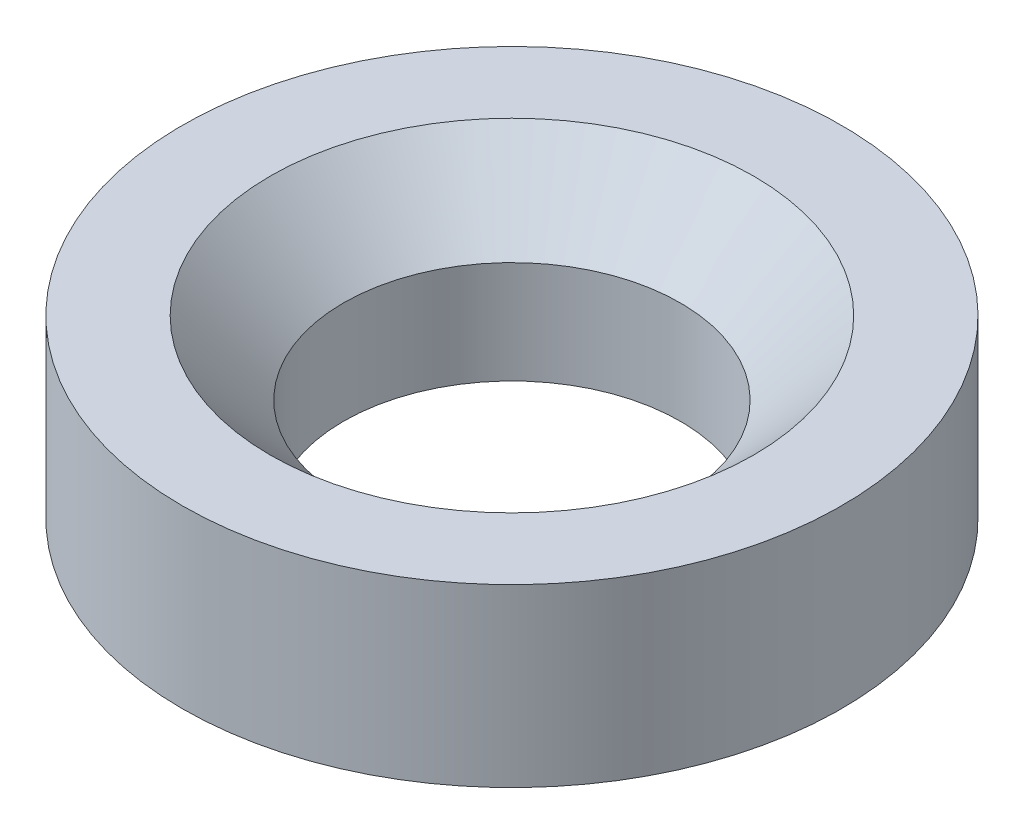
ISO-10303-21;
HEADER;
FILE_DESCRIPTION(('STEP AP214'),'2;1');
FILE_NAME('part.step','',(''),(''),'','','');
FILE_SCHEMA(('AUTOMOTIVE_DESIGN { 1 0 10303 214 1 1 1 1 }'));
ENDSEC;
DATA;
#1=APPLICATION_CONTEXT('core data for automotive mechanical design processes');
#2=APPLICATION_PROTOCOL_DEFINITION('international standard','automotive_design',2000,#1);
#3=PRODUCT_CONTEXT('',#1,'mechanical');
#4=PRODUCT('Part','Part','',(#3));
#5=PRODUCT_RELATED_PRODUCT_CATEGORY('part','',(#4));
#6=PRODUCT_DEFINITION_FORMATION('','',#4);
#7=PRODUCT_DEFINITION_CONTEXT('part definition',#1,'design');
#8=PRODUCT_DEFINITION('design','',#6,#7);
#9=PRODUCT_DEFINITION_SHAPE('','',#8);
#10=(LENGTH_UNIT() NAMED_UNIT(*) SI_UNIT(.MILLI.,.METRE.));
#11=(NAMED_UNIT(*) PLANE_ANGLE_UNIT() SI_UNIT($,.RADIAN.));
#12=(NAMED_UNIT(*) SI_UNIT($,.STERADIAN.) SOLID_ANGLE_UNIT());
#13=UNCERTAINTY_MEASURE_WITH_UNIT(LENGTH_MEASURE(1.E-05),#10,'distance_accuracy_value','');
#14=(GEOMETRIC_REPRESENTATION_CONTEXT(3) GLOBAL_UNCERTAINTY_ASSIGNED_CONTEXT((#13)) GLOBAL_UNIT_ASSIGNED_CONTEXT((#10,
#11,#12)) REPRESENTATION_CONTEXT('',''));
#15=CARTESIAN_POINT('',(0.,0.,0.));
#16=DIRECTION('',(0.,0.,1.));
#17=DIRECTION('',(1.,0.,0.));
#18=AXIS2_PLACEMENT_3D('',#15,#16,#17);
#19=CARTESIAN_POINT('',(0.,12.,0.));
#20=DIRECTION('',(0.,-1.,0.));
#21=DIRECTION('',(0.,0.,-1.));
#22=AXIS2_PLACEMENT_3D('',#19,#20,#21);
#23=CYLINDRICAL_SURFACE('',#22,22.5);
#24=CARTESIAN_POINT('',(0.,12.,0.));
#25=DIRECTION('',(0.,1.,0.));
#26=DIRECTION('',(0.,0.,1.));
#27=AXIS2_PLACEMENT_3D('',#24,#25,#26);
#28=CIRCLE('',#27,22.5);
#29=CARTESIAN_POINT('',(0.,12.,22.5));
#30=VERTEX_POINT('',#29);
#31=EDGE_CURVE('E10',#30,#30,#28,.T.);
#32=ORIENTED_EDGE('',*,*,#31,.F.);
#33=EDGE_LOOP('',(#32));
#34=FACE_BOUND('',#33,.T.);
#35=CARTESIAN_POINT('',(0.,0.,0.));
#36=DIRECTION('',(0.,1.,0.));
#37=DIRECTION('',(0.,0.,1.));
#38=AXIS2_PLACEMENT_3D('',#35,#36,#37);
#39=CIRCLE('',#38,22.5);
#40=CARTESIAN_POINT('',(0.,0.,22.5));
#41=VERTEX_POINT('',#40);
#42=EDGE_CURVE('E37',#41,#41,#39,.T.);
#43=ORIENTED_EDGE('',*,*,#42,.T.);
#44=EDGE_LOOP('',(#43));
#45=FACE_BOUND('',#44,.T.);
#46=ADVANCED_FACE('F40',(#34,#45),#23,.T.);
#47=CARTESIAN_POINT('',(0.,12.,0.));
#48=DIRECTION('',(0.,1.,0.));
#49=DIRECTION('',(0.,0.,1.));
#50=AXIS2_PLACEMENT_3D('',#47,#48,#49);
#51=PLANE('',#50);
#52=CARTESIAN_POINT('',(0.,12.,0.));
#53=DIRECTION('',(0.,1.,0.));
#54=DIRECTION('',(-1.,0.,0.));
#55=AXIS2_PLACEMENT_3D('',#52,#53,#54);
#56=CIRCLE('',#55,16.5);
#57=CARTESIAN_POINT('',(-16.5,12.,0.));
#58=VERTEX_POINT('',#57);
#59=EDGE_CURVE('E53',#58,#58,#56,.T.);
#60=ORIENTED_EDGE('',*,*,#59,.F.);
#61=EDGE_LOOP('',(#60));
#62=FACE_BOUND('',#61,.T.);
#63=ORIENTED_EDGE('',*,*,#31,.T.);
#64=EDGE_LOOP('',(#63));
#65=FACE_BOUND('',#64,.T.);
#66=ADVANCED_FACE('F61',(#62,#65),#51,.T.);
#67=CARTESIAN_POINT('',(0.,0.,0.));
#68=DIRECTION('',(0.,1.,0.));
#69=DIRECTION('',(0.,0.,1.));
#70=AXIS2_PLACEMENT_3D('',#67,#68,#69);
#71=PLANE('',#70);
#72=CARTESIAN_POINT('',(0.,0.,0.));
#73=DIRECTION('',(0.,1.,0.));
#74=DIRECTION('',(-1.,0.,0.));
#75=AXIS2_PLACEMENT_3D('',#72,#73,#74);
#76=CIRCLE('',#75,11.5);
#77=CARTESIAN_POINT('',(-11.5,0.,0.));
#78=VERTEX_POINT('',#77);
#79=EDGE_CURVE('E50',#78,#78,#76,.T.);
#80=ORIENTED_EDGE('',*,*,#79,.T.);
#81=EDGE_LOOP('',(#80));
#82=FACE_BOUND('',#81,.T.);
#83=ORIENTED_EDGE('',*,*,#42,.F.);
#84=EDGE_LOOP('',(#83));
#85=FACE_BOUND('',#84,.T.);
#86=ADVANCED_FACE('F64',(#82,#85),#71,.F.);
#87=CARTESIAN_POINT('',(0.,12.,0.));
#88=DIRECTION('',(0.,1.,0.));
#89=DIRECTION('',(-1.,0.,0.));
#90=AXIS2_PLACEMENT_3D('',#87,#88,#89);
#91=CYLINDRICAL_SURFACE('',#90,11.5);
#92=CARTESIAN_POINT('',(0.,7.00000000000003,0.));
#93=DIRECTION('',(0.,1.,0.));
#94=DIRECTION('',(-1.,0.,0.));
#95=AXIS2_PLACEMENT_3D('',#92,#93,#94);
#96=CIRCLE('',#95,11.5);
#97=CARTESIAN_POINT('',(-11.5,7.00000000000004,0.));
#98=VERTEX_POINT('',#97);
#99=EDGE_CURVE('E51',#98,#98,#96,.T.);
#100=ORIENTED_EDGE('',*,*,#99,.T.);
#101=EDGE_LOOP('',(#100));
#102=FACE_BOUND('',#101,.T.);
#103=ORIENTED_EDGE('',*,*,#79,.F.);
#104=EDGE_LOOP('',(#103));
#105=FACE_BOUND('',#104,.T.);
#106=ADVANCED_FACE('F69',(#102,#105),#91,.F.);
#107=CARTESIAN_POINT('',(0.,7.00000000000003,0.));
#108=DIRECTION('',(0.,1.,0.));
#109=DIRECTION('',(-1.,0.,0.));
#110=AXIS2_PLACEMENT_3D('',#107,#108,#109);
#111=CONICAL_SURFACE('',#110,11.5,0.78539816339745);
#112=ORIENTED_EDGE('',*,*,#59,.T.);
#113=EDGE_LOOP('',(#112));
#114=FACE_BOUND('',#113,.T.);
#115=ORIENTED_EDGE('',*,*,#99,.F.);
#116=EDGE_LOOP('',(#115));
#117=FACE_BOUND('',#116,.T.);
#118=ADVANCED_FACE('F59',(#114,#117),#111,.F.);
#119=CLOSED_SHELL('',(#46,#66,#86,#106,#118));
#120=MANIFOLD_SOLID_BREP('B2',#119);
#121=ADVANCED_BREP_SHAPE_REPRESENTATION('',(#18,#120),#14);
#122=SHAPE_DEFINITION_REPRESENTATION(#9,#121);
ENDSEC;
END-ISO-10303-21;
